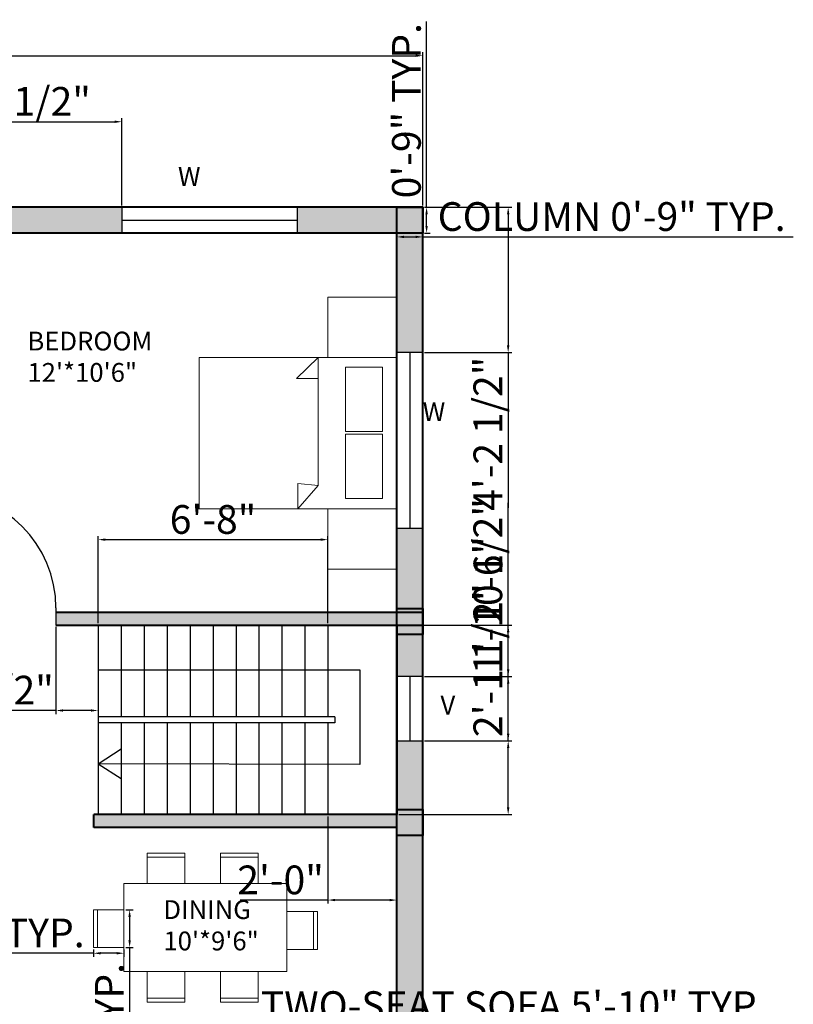
# Model space of a CAD drawing. Units: inches. Extents: x 1628 to 2197, y 2073 to 2736.
# Tile 3 of 3: x 1913 to 2182, y 2323 to 2666. Entities that reach past the tile are written whole.
import ezdxf

# ---------------------------------------------------------------- set-up
doc = ezdxf.new("R2010")
doc.units = ezdxf.units.IN
for name, color, linetype, lineweight in [('A-ANNO-DIMS', 2, 'Continuous', 18), ('A-ANNO-IDEN', 7, 'Continuous', 18), ('A-AREA-IDEN', 7, 'Continuous', 18), ('A-COLS', 7, 'Continuous', 40), ('A-COLS-PATT', 8, 'Continuous', 13), ('A-FLOR-STRS', 7, 'Continuous', 25), ('A-FURN', 8, 'Continuous', 18), ('A-WALL-PATT', 152, 'Continuous', 13), ('bed', 210, 'Continuous', 18), ('door', 52, 'Continuous', 25), ('wall', 151, 'Continuous', 40), ('window', 20, 'Continuous', 25)]:
    doc.layers.add(name, color=color, linetype=linetype, lineweight=lineweight)
doc.styles.get("Standard").update_dxf_attribs({"font": 'arial.ttf'})
doc.dimstyles.new('ISO-25', dxfattribs={"dimtxt": 10, "dimasz": 2.5, "dimexe": 1.25, "dimexo": 0.625, "dimtad": 1, "dimdec": 0, "dimlunit": 4, "dimtxsty": 'Standard', "dimcen": 2.5, "dimadec": 0, "dimazin": 0, "dimtfac": 1, "dimtdec": 0, "dimtmove": 0, "dimatfit": 3, "dimfxl": 1, "dimarcsym": 0})

# ---------------------------------------------------------------- blocks, each defined once
blk = doc.blocks.new('*U2')
for p, q in [((0, 0), (0, -6)), ((40, 0), (40, -6))]:
    blk.add_line(p, q)
blk.add_lwpolyline([(0, 0), (0, 40), (1.75, 40), (1.75, 0)], close=True)
blk.add_arc((0, 0), 40, 0, 90)
blk = doc.blocks.new('*D5')
at = {"layer": 'A-ANNO-DIMS', "color": 0, "lineweight": -2, "transparency": 16777216}
for p, q in [((1693.11, 2601.33), (1693.11, 2654.69)), ((2053.11, 2601.33), (2053.11, 2654.69)), ((1695.61, 2653.44), (2050.61, 2653.44))]:
    blk.add_line(p, q, dxfattribs=at)
at = {"layer": 'A-ANNO-DIMS', "color": 0, "transparency": 16777216}
for points in [[(1695.61, 2653.85), (1695.61, 2653.02), (1693.11, 2653.44)], [(2050.61, 2653.85), (2050.61, 2653.02), (2053.11, 2653.44)]]:
    blk.add_solid(points, dxfattribs=at)
at = {"layer": 'Defpoints', "color": 0, "transparency": 16777216}
for p in [(2053.11, 2653.44), (1693.11, 2600.7), (2053.11, 2600.7)]:
    blk.add_point(p, dxfattribs=at)
at = {"layer": 'A-ANNO-DIMS', "color": 0, "transparency": 16777216, "insert": (1873.11, 2659.17), "char_height": 10, "attachment_point": 5}
blk.add_mtext("30'", dxfattribs=at)
blk = doc.blocks.new('BED-DOUBLE-WITH-NIGHTSTANDS')
for p, q in [((27.37, 65.6), (34.42, 73.72)), ((34.42, 73.72), (34.42, 64.86)), ((27.37, 28.24), (27.37, 65.6)), ((34.42, 64.86), (27.37, 65.6)), ((27.37, 28.24), (27.37, 20.94)), ((27.37, 20.94), (34.96, 28.24)), ((34.96, 28.24), (27.37, 28.24))]:
    blk.add_line(p, q)
for points in [[(0, 73.72), (23.98, 73.72), (23.98, 94.66), (0, 94.66)], [(0, 20.94), (68.84, 20.94), (68.84, 73.72), (0, 73.72)], [(4.97, 47.66), (17.93, 47.66), (17.93, 70.03), (4.97, 70.03)], [(4.97, 24.36), (17.93, 24.36), (17.93, 46.73), (4.97, 46.73)], [(0, 0), (23.98, 0), (23.98, 20.94), (0, 20.94)]]:
    blk.add_lwpolyline(points, close=True)
blk = doc.blocks.new('CHAIR-DINING')
for p, q in [((1.86, 9.22), (0, 9.22)), ((0, 9.22), (13.17, 9.22))]:
    blk.add_line(p, q)
blk.add_lwpolyline([(0, 0), (13.17, 0), (13.17, 10.6), (0, 10.6)], close=True)
blk = doc.blocks.new('WINDOW-61IN')
blk.add_line((0, 4.5), (61.1, 4.5))
blk.add_lwpolyline([(0, 0), (61.1, 0), (61.1, 9), (0, 9)], close=True)
blk = doc.blocks.new('COLUMN-9X9')
blk.add_lwpolyline([(0, 9), (9, 9), (9, 0), (0, 0)], close=True)
blk = doc.blocks.new('*D13')
at = {"layer": 'A-ANNO-DIMS', "color": 0, "lineweight": -2, "transparency": 16777216}
for p, q in [((2044.11, 2591.08), (2044.11, 2589.1)), ((2046.61, 2590.35), (2050.61, 2590.35)), ((2053.11, 2591.08), (2053.11, 2589.1)), ((2053.11, 2590.35), (2182.12, 2590.35))]:
    blk.add_line(p, q, dxfattribs=at)
at = {"layer": 'A-ANNO-DIMS', "color": 0, "transparency": 16777216}
for points in [[(2046.61, 2590.77), (2046.61, 2589.94), (2044.11, 2590.35)], [(2050.61, 2590.77), (2050.61, 2589.94), (2053.11, 2590.35)]]:
    blk.add_solid(points, dxfattribs=at)
at = {"layer": 'Defpoints', "color": 0, "transparency": 16777216}
for p in [(2044.11, 2591.7), (2053.11, 2591.7), (2053.11, 2590.35)]:
    blk.add_point(p, dxfattribs=at)
at = {"layer": 'A-ANNO-DIMS', "color": 0, "transparency": 16777216, "insert": (2118.87, 2596.15), "char_height": 10, "attachment_point": 5}
blk.add_mtext('COLUMN 0\'-9" TYP.', dxfattribs=at)
blk = doc.blocks.new('*D14')
at = {"layer": 'A-ANNO-DIMS', "color": 0, "lineweight": -2, "transparency": 16777216}
for p, q in [((2054.46, 2600.7), (2054.46, 2665.41)), ((2053.74, 2600.7), (2055.71, 2600.7)), ((2054.46, 2594.2), (2054.46, 2598.2)), ((2053.74, 2591.7), (2055.71, 2591.7))]:
    blk.add_line(p, q, dxfattribs=at)
at = {"layer": 'A-ANNO-DIMS', "color": 0, "transparency": 16777216}
for points in [[(2054.04, 2598.2), (2054.88, 2598.2), (2054.46, 2600.7)], [(2054.04, 2594.2), (2054.88, 2594.2), (2054.46, 2591.7)]]:
    blk.add_solid(points, dxfattribs=at)
at = {"layer": 'Defpoints', "color": 0, "transparency": 16777216}
for p in [(2053.11, 2600.7), (2054.46, 2600.7), (2053.11, 2591.7)]:
    blk.add_point(p, dxfattribs=at)
at = {"layer": 'A-ANNO-DIMS', "color": 0, "transparency": 16777216, "insert": (2048.73, 2634.3), "char_height": 10, "attachment_point": 5, "rotation": 90}
blk.add_mtext('0\'-9" TYP.', dxfattribs=at)
blk = doc.blocks.new('*D17')
at = {"layer": 'A-ANNO-DIMS', "color": 0, "lineweight": -2, "transparency": 16777216}
for p, q in [((1949.73, 2356.08), (1952.33, 2356.08)), ((1951.08, 2353.58), (1951.08, 2345.41)), ((1949.73, 2342.91), (1952.33, 2342.91)), ((1951.08, 2342.91), (1951.08, 2230.98))]:
    blk.add_line(p, q, dxfattribs=at)
at = {"layer": 'A-ANNO-DIMS', "color": 0, "transparency": 16777216}
for points in [[(1950.66, 2353.58), (1951.5, 2353.58), (1951.08, 2356.08)], [(1950.66, 2345.41), (1951.5, 2345.41), (1951.08, 2342.91)]]:
    blk.add_solid(points, dxfattribs=at)
at = {"layer": 'Defpoints', "color": 0, "transparency": 16777216}
for p in [(1949.11, 2356.08), (1949.11, 2342.91), (1951.08, 2342.91)]:
    blk.add_point(p, dxfattribs=at)
at = {"layer": 'A-ANNO-DIMS', "color": 0, "transparency": 16777216, "insert": (1945.29, 2285.7), "char_height": 10, "attachment_point": 5, "rotation": 90}
blk.add_mtext('CHAIR 1\'-1" TYP.', dxfattribs=at)
blk = doc.blocks.new('*D18')
at = {"layer": 'A-ANNO-DIMS', "color": 0, "lineweight": -2, "transparency": 16777216}
for p, q in [((1938.5, 2342.29), (1938.5, 2339.69)), ((1949.11, 2342.29), (1949.11, 2339.69)), ((1938.5, 2340.94), (1842.73, 2340.94)), ((1946.61, 2340.94), (1941, 2340.94))]:
    blk.add_line(p, q, dxfattribs=at)
at = {"layer": 'A-ANNO-DIMS', "color": 0, "transparency": 16777216}
for points in [[(1941, 2341.35), (1941, 2340.52), (1938.5, 2340.94)], [(1946.61, 2341.35), (1946.61, 2340.52), (1949.11, 2340.94)]]:
    blk.add_solid(points, dxfattribs=at)
at = {"layer": 'Defpoints', "color": 0, "transparency": 16777216}
for p in [(1938.5, 2342.91), (1949.11, 2342.91), (1938.5, 2340.94)]:
    blk.add_point(p, dxfattribs=at)
at = {"layer": 'A-ANNO-DIMS', "color": 0, "transparency": 16777216, "insert": (1889.36, 2346.73), "char_height": 10, "attachment_point": 5}
blk.add_mtext('0\'-10 1/2" TYP.', dxfattribs=at)
blk = doc.blocks.new('*D23')
at = {"layer": 'A-ANNO-DIMS', "color": 0, "lineweight": -2, "transparency": 16777216}
for p, q in [((1917.57, 2305.72), (1917.57, 2316.85)), ((1920.07, 2315.6), (1985.07, 2315.6)), ((1987.57, 2305.72), (1987.57, 2316.85)), ((1987.57, 2315.6), (2179.82, 2315.6))]:
    blk.add_line(p, q, dxfattribs=at)
at = {"layer": 'A-ANNO-DIMS', "color": 0, "transparency": 16777216}
for points in [[(1920.07, 2316.01), (1920.07, 2315.18), (1917.57, 2315.6)], [(1985.07, 2316.01), (1985.07, 2315.18), (1987.57, 2315.6)]]:
    blk.add_solid(points, dxfattribs=at)
at = {"layer": 'Defpoints', "color": 0, "transparency": 16777216}
for p in [(1987.57, 2315.6), (1917.57, 2305.1), (1987.57, 2305.1)]:
    blk.add_point(p, dxfattribs=at)
at = {"layer": 'A-ANNO-DIMS', "color": 0, "transparency": 16777216, "insert": (2084.94, 2321.4), "char_height": 10, "attachment_point": 5}
blk.add_mtext('TWO-SEAT SOFA 5\'-10" TYP.', dxfattribs=at)
blk = doc.blocks.new('*D24')
at = {"layer": 'A-ANNO-DIMS', "color": 0, "lineweight": -2, "transparency": 16777216}
for p, q in [((1907.07, 2305.1), (1907.07, 2393.27)), ((1916.95, 2305.1), (1905.82, 2305.1)), ((1907.07, 2274.24), (1907.07, 2302.6)), ((1916.95, 2271.74), (1905.82, 2271.74))]:
    blk.add_line(p, q, dxfattribs=at)
at = {"layer": 'A-ANNO-DIMS', "color": 0, "transparency": 16777216}
for points in [[(1906.65, 2302.6), (1907.49, 2302.6), (1907.07, 2305.1)], [(1906.65, 2274.24), (1907.49, 2274.24), (1907.07, 2271.74)]]:
    blk.add_solid(points, dxfattribs=at)
at = {"layer": 'Defpoints', "color": 0, "transparency": 16777216}
for p in [(1907.07, 2305.1), (1917.57, 2305.1), (1917.57, 2271.74)]:
    blk.add_point(p, dxfattribs=at)
at = {"layer": 'A-ANNO-DIMS', "color": 0, "transparency": 16777216, "insert": (1901.28, 2350.44), "char_height": 10, "attachment_point": 5, "rotation": 90}
blk.add_mtext('2\'-9 1/2" TYP.', dxfattribs=at)
blk = doc.blocks.new('*D27')
at = {"layer": 'A-ANNO-DIMS', "color": 0, "lineweight": -2, "transparency": 16777216}
for p, q in [((1873.11, 2592.33), (1873.11, 2631.7)), ((1875.61, 2630.45), (1945.87, 2630.45)), ((1948.37, 2601.33), (1948.37, 2631.7))]:
    blk.add_line(p, q, dxfattribs=at)
at = {"layer": 'A-ANNO-DIMS', "color": 0, "transparency": 16777216}
for points in [[(1875.61, 2630.87), (1875.61, 2630.04), (1873.11, 2630.45)], [(1945.87, 2630.87), (1945.87, 2630.04), (1948.37, 2630.45)]]:
    blk.add_solid(points, dxfattribs=at)
at = {"layer": 'Defpoints', "color": 0, "transparency": 16777216}
for p in [(1948.37, 2630.45), (1948.37, 2600.7), (1873.11, 2591.7)]:
    blk.add_point(p, dxfattribs=at)
at = {"layer": 'A-ANNO-DIMS', "color": 0, "transparency": 16777216, "insert": (1910.74, 2636.25), "char_height": 10, "attachment_point": 5}
blk.add_mtext('6\'-3 1/2"', dxfattribs=at)
blk = doc.blocks.new('*D42')
at = {"layer": 'A-ANNO-DIMS', "color": 0, "lineweight": -2, "transparency": 16777216}
for p, q in [((2053.74, 2600.7), (2084.11, 2600.7)), ((2082.86, 2598.2), (2082.86, 2552.57)), ((2053.74, 2550.07), (2084.11, 2550.07)), ((2082.86, 2550.07), (2082.86, 2496.04))]:
    blk.add_line(p, q, dxfattribs=at)
at = {"layer": 'A-ANNO-DIMS', "color": 0, "transparency": 16777216}
for points in [[(2082.44, 2598.2), (2083.28, 2598.2), (2082.86, 2600.7)], [(2082.44, 2552.57), (2083.28, 2552.57), (2082.86, 2550.07)]]:
    blk.add_solid(points, dxfattribs=at)
at = {"layer": 'Defpoints', "color": 0, "transparency": 16777216}
for p in [(2053.11, 2600.7), (2053.11, 2550.07), (2082.86, 2550.07)]:
    blk.add_point(p, dxfattribs=at)
at = {"layer": 'A-ANNO-DIMS', "color": 0, "transparency": 16777216, "insert": (2077.07, 2521.8), "char_height": 10, "attachment_point": 5, "rotation": 90}
blk.add_mtext('4\'-2 1/2"', dxfattribs=at)
blk = doc.blocks.new('*D43')
at = {"layer": 'A-ANNO-DIMS', "color": 0, "lineweight": -2, "transparency": 16777216}
for p, q in [((2082.86, 2414.88), (2082.86, 2468.69)), ((2053.74, 2414.88), (2084.11, 2414.88)), ((2082.86, 2391.7), (2082.86, 2412.38)), ((2044.74, 2389.2), (2084.11, 2389.2))]:
    blk.add_line(p, q, dxfattribs=at)
at = {"layer": 'A-ANNO-DIMS', "color": 0, "transparency": 16777216}
for points in [[(2082.44, 2412.38), (2083.28, 2412.38), (2082.86, 2414.88)], [(2082.44, 2391.7), (2083.28, 2391.7), (2082.86, 2389.2)]]:
    blk.add_solid(points, dxfattribs=at)
at = {"layer": 'Defpoints', "color": 0, "transparency": 16777216}
for p in [(2053.11, 2414.88), (2082.86, 2414.88), (2044.11, 2389.2)]:
    blk.add_point(p, dxfattribs=at)
at = {"layer": 'A-ANNO-DIMS', "color": 0, "transparency": 16777216, "insert": (2077.07, 2443.03), "char_height": 10, "attachment_point": 5, "rotation": 90}
blk.add_mtext('2\'-1 1/2"', dxfattribs=at)
blk = doc.blocks.new('*D44')
at = {"layer": 'A-ANNO-DIMS', "color": 0, "lineweight": -2, "transparency": 16777216}
for p, q in [((2082.86, 2437.29), (2082.86, 2497.75)), ((2053.74, 2437.29), (2084.11, 2437.29)), ((2082.86, 2417.38), (2082.86, 2434.79)), ((2053.74, 2414.88), (2084.11, 2414.88))]:
    blk.add_line(p, q, dxfattribs=at)
at = {"layer": 'A-ANNO-DIMS', "color": 0, "transparency": 16777216}
for points in [[(2082.44, 2434.79), (2083.28, 2434.79), (2082.86, 2437.29)], [(2082.44, 2417.38), (2083.28, 2417.38), (2082.86, 2414.88)]]:
    blk.add_solid(points, dxfattribs=at)
at = {"layer": 'Defpoints', "color": 0, "transparency": 16777216}
for p in [(2053.11, 2437.29), (2082.86, 2437.29), (2053.11, 2414.88)]:
    blk.add_point(p, dxfattribs=at)
at = {"layer": 'A-ANNO-DIMS', "color": 0, "transparency": 16777216, "insert": (2077.07, 2468.77), "char_height": 10, "attachment_point": 5, "rotation": 90}
blk.add_mtext('1\'-10 1/2"', dxfattribs=at)
blk = doc.blocks.new('*D45')
at = {"layer": 'A-ANNO-DIMS', "color": 0, "lineweight": -2, "transparency": 16777216}
for p, q in [((2082.86, 2455.2), (2082.86, 2484.59)), ((2044.74, 2455.2), (2084.11, 2455.2)), ((2082.86, 2439.79), (2082.86, 2452.7)), ((2053.74, 2437.29), (2084.11, 2437.29))]:
    blk.add_line(p, q, dxfattribs=at)
at = {"layer": 'A-ANNO-DIMS', "color": 0, "transparency": 16777216}
for points in [[(2082.44, 2452.7), (2083.28, 2452.7), (2082.86, 2455.2)], [(2082.44, 2439.79), (2083.28, 2439.79), (2082.86, 2437.29)]]:
    blk.add_solid(points, dxfattribs=at)
at = {"layer": 'Defpoints', "color": 0, "transparency": 16777216}
for p in [(2044.11, 2455.2), (2082.86, 2455.2), (2053.11, 2437.29)]:
    blk.add_point(p, dxfattribs=at)
at = {"layer": 'A-ANNO-DIMS', "color": 0, "transparency": 16777216, "insert": (2077.13, 2471.15), "char_height": 10, "attachment_point": 5, "rotation": 90}
blk.add_mtext('1\'-6"', dxfattribs=at)
blk = doc.blocks.new('*D46')
at = {"layer": 'A-ANNO-DIMS', "color": 0, "lineweight": -2, "transparency": 16777216}
for p, q in [((1940.11, 2455.83), (1940.11, 2486.2)), ((2020.11, 2455.83), (2020.11, 2486.2)), ((1942.61, 2484.95), (2017.61, 2484.95))]:
    blk.add_line(p, q, dxfattribs=at)
at = {"layer": 'A-ANNO-DIMS', "color": 0, "transparency": 16777216}
for points in [[(1942.61, 2485.37), (1942.61, 2484.54), (1940.11, 2484.95)], [(2017.61, 2485.37), (2017.61, 2484.54), (2020.11, 2484.95)]]:
    blk.add_solid(points, dxfattribs=at)
at = {"layer": 'Defpoints', "color": 0, "transparency": 16777216}
for p in [(2020.11, 2484.95), (1940.11, 2455.2), (2020.11, 2455.2)]:
    blk.add_point(p, dxfattribs=at)
at = {"layer": 'A-ANNO-DIMS', "color": 0, "transparency": 16777216, "insert": (1980.11, 2490.68), "char_height": 10, "attachment_point": 5}
blk.add_mtext('6\'-8"', dxfattribs=at)
blk = doc.blocks.new('*D47')
at = {"layer": 'A-ANNO-DIMS', "color": 0, "lineweight": -2, "transparency": 16777216}
for p, q in [((2020.11, 2388.58), (2020.11, 2358.2)), ((2044.11, 2388.58), (2044.11, 2358.2)), ((2020.11, 2359.45), (1989.61, 2359.45)), ((2041.61, 2359.45), (2022.61, 2359.45))]:
    blk.add_line(p, q, dxfattribs=at)
at = {"layer": 'A-ANNO-DIMS', "color": 0, "transparency": 16777216}
for points in [[(2022.61, 2359.87), (2022.61, 2359.04), (2020.11, 2359.45)], [(2041.61, 2359.87), (2041.61, 2359.04), (2044.11, 2359.45)]]:
    blk.add_solid(points, dxfattribs=at)
at = {"layer": 'Defpoints', "color": 0, "transparency": 16777216}
for p in [(2020.11, 2389.2), (2044.11, 2389.2), (2020.11, 2359.45)]:
    blk.add_point(p, dxfattribs=at)
at = {"layer": 'A-ANNO-DIMS', "color": 0, "transparency": 16777216, "insert": (2003.61, 2365.18), "char_height": 10, "attachment_point": 5}
blk.add_mtext('2\'-0"', dxfattribs=at)
blk = doc.blocks.new('*D51')
at = {"layer": 'A-ANNO-DIMS', "color": 0, "lineweight": -2, "transparency": 16777216}
for p, q in [((1925.43, 2454.58), (1925.43, 2424.2)), ((1940.11, 2454.58), (1940.11, 2424.2)), ((1925.43, 2425.45), (1872.74, 2425.45)), ((1937.61, 2425.45), (1927.93, 2425.45))]:
    blk.add_line(p, q, dxfattribs=at)
at = {"layer": 'A-ANNO-DIMS', "color": 0, "transparency": 16777216}
for points in [[(1927.93, 2425.87), (1927.93, 2425.04), (1925.43, 2425.45)], [(1937.61, 2425.87), (1937.61, 2425.04), (1940.11, 2425.45)]]:
    blk.add_solid(points, dxfattribs=at)
at = {"layer": 'Defpoints', "color": 0, "transparency": 16777216}
for p in [(1925.43, 2455.2), (1940.11, 2455.2), (1925.43, 2425.45)]:
    blk.add_point(p, dxfattribs=at)
at = {"layer": 'A-ANNO-DIMS', "color": 0, "transparency": 16777216, "insert": (1897.84, 2431.25), "char_height": 10, "attachment_point": 5}
blk.add_mtext('1\'-2 1/2"', dxfattribs=at)

msp = doc.modelspace()

# ---------------------------------------------------------------- hatches: boundary and pattern name
at = {"layer": 'A-COLS-PATT'}
h = msp.add_hatch(color=256, dxfattribs=at)
h.dxf.hatch_style = 1
h.paths.add_polyline_path([(1702.11, 2600.7), (1693.11, 2600.7), (1693.11, 2591.7), (1702.11, 2591.7)])
h.paths.add_polyline_path([(1879.79, 2600.7), (1870.79, 2600.7), (1870.79, 2591.7), (1879.79, 2591.7)])
h.paths.add_polyline_path([(2053.11, 2600.7), (2044.11, 2600.7), (2044.11, 2591.7), (2053.11, 2591.7)])
h.paths.add_polyline_path([(1702.11, 2395.2), (1693.11, 2395.2), (1693.11, 2386.2), (1702.11, 2386.2)])
h.paths.add_polyline_path([(1826.61, 2395.2), (1817.61, 2395.2), (1817.61, 2386.2), (1826.61, 2386.2)])
h.paths.add_polyline_path([(1702.11, 2459.7), (1693.11, 2459.7), (1693.11, 2450.7), (1702.11, 2450.7)])
h.paths.add_polyline_path([(2053.11, 2459.7), (2044.11, 2459.7), (2044.11, 2455.2), (2053.11, 2455.2)])
h.paths.add_polyline_path([(2053.11, 2455.2), (2044.11, 2455.2), (2044.11, 2451.94), (2053.11, 2451.94)])
h.paths.add_polyline_path([(2053.11, 2460.94), (2044.11, 2460.94), (2044.11, 2459.7), (2053.11, 2459.7)])
h.paths.add_polyline_path([(2053.11, 2390.99), (2044.11, 2390.99), (2044.11, 2381.99), (2053.11, 2381.99)])
h.paths.add_polyline_path([(2053.11, 2322.52), (2044.11, 2322.52), (2044.11, 2313.52), (2053.11, 2313.52)])
h.paths.add_polyline_path([(1702.11, 2294.7), (1693.11, 2294.7), (1693.11, 2285.7), (1702.11, 2285.7)])
h.paths.add_polyline_path([(1702.11, 2129.7), (1693.11, 2129.7), (1693.11, 2120.7), (1702.11, 2120.7)])
h.paths.add_polyline_path([(1831.35, 2129.7), (1822.35, 2129.7), (1822.35, 2120.7), (1831.35, 2120.7)])
h.paths.add_polyline_path([(1883.72, 2129.7), (1874.72, 2129.7), (1874.72, 2120.7), (1883.72, 2120.7)])
h.paths.add_polyline_path([(2053.11, 2129.7), (2044.11, 2129.7), (2044.11, 2120.7), (2053.11, 2120.7)])
at = {"layer": 'A-WALL-PATT'}
h = msp.add_hatch(color=256, dxfattribs=at)
h.dxf.hatch_style = 1
h.paths.add_polyline_path([(1753.01, 2600.7), (1702.11, 2600.7), (1702.11, 2591.7), (1753.01, 2591.7)])
h.paths.add_polyline_path([(1870.79, 2600.7), (1814.12, 2600.7), (1814.12, 2591.7), (1870.79, 2591.7)])
h.paths.add_polyline_path([(1948.37, 2600.7), (1879.79, 2600.7), (1879.79, 2591.7), (1909.32, 2591.7), (1948.37, 2591.7)])
h.paths.add_polyline_path([(2044.11, 2600.7), (2009.47, 2600.7), (2009.47, 2591.7), (2044.11, 2591.7)])
h.paths.add_polyline_path([(2053.11, 2591.7), (2044.11, 2591.7), (2044.11, 2550.07), (2053.11, 2550.07)])
h.paths.add_polyline_path([(1702.11, 2591.7), (1693.11, 2591.7), (1693.11, 2549.95), (1702.11, 2549.95)])
h.paths.add_polyline_path([(1702.11, 2488.85), (1693.11, 2488.85), (1693.11, 2459.7), (1702.11, 2459.7)])
h.paths.add_polyline_path([(1828.05, 2459.7), (1702.11, 2459.7), (1702.11, 2455.2), (1733.61, 2455.2), (1792.11, 2455.2), (1828.05, 2455.2)])
h.paths.add_polyline_path([(1885.43, 2459.7), (1868.05, 2459.7), (1868.05, 2455.2), (1885.43, 2455.2)])
h.paths.add_polyline_path([(2053.11, 2488.97), (2044.11, 2488.97), (2044.11, 2474.68), (2044.11, 2460.94), (2053.11, 2460.94)])
h.paths.add_polyline_path([(2053.11, 2451.94), (2044.11, 2451.94), (2044.11, 2437.29), (2053.11, 2437.29)])
h.paths.add_polyline_path([(2053.11, 2414.88), (2044.11, 2414.88), (2044.11, 2390.99), (2053.11, 2390.99)])
h.paths.add_polyline_path([(2044.11, 2459.7), (1925.43, 2459.7), (1925.43, 2455.2), (2044.11, 2455.2)])
h.paths.add_polyline_path([(2053.11, 2381.99), (2044.11, 2381.99), (2044.11, 2322.52), (2053.11, 2322.52)])
h.paths.add_polyline_path([(1919.51, 2129.7), (1883.72, 2129.7), (1883.72, 2120.7), (1919.51, 2120.7)])
h.paths.add_polyline_path([(2044.11, 2129.7), (1980.61, 2129.7), (1980.61, 2120.7), (2044.11, 2120.7)])
h.paths.add_polyline_path([(2053.11, 2207.91), (2044.11, 2207.91), (2044.11, 2129.7), (2053.11, 2129.7)])
h.paths.add_polyline_path([(2053.11, 2313.52), (2044.11, 2313.52), (2044.11, 2269.02), (2053.11, 2269.02)])
h.paths.add_polyline_path([(1822.35, 2129.7), (1785.25, 2129.7), (1785.25, 2120.7), (1822.35, 2120.7)])
h.paths.add_polyline_path([(1724.14, 2129.7), (1702.11, 2129.7), (1702.11, 2120.7), (1724.14, 2120.7)])
h.paths.add_polyline_path([(1702.11, 2168.74), (1693.11, 2168.74), (1693.11, 2129.7), (1702.11, 2129.7)])
h.paths.add_polyline_path([(1702.11, 2285.7), (1693.11, 2285.7), (1693.11, 2229.84), (1702.11, 2229.84)])
h.paths.add_polyline_path([(1702.11, 2317.65), (1693.11, 2317.65), (1693.11, 2294.7), (1702.11, 2294.7)])
h.paths.add_polyline_path([(1702.11, 2386.2), (1693.11, 2386.2), (1693.11, 2378.75), (1702.11, 2378.75)])
h.paths.add_polyline_path([(2044.11, 2389.2), (1938.65, 2389.2), (1938.65, 2384.7), (2044.11, 2384.7)])
h.paths.add_polyline_path([(1817.61, 2395.2), (1782.07, 2395.2), (1702.11, 2395.2), (1702.11, 2390.7), (1796.61, 2390.7), (1817.61, 2390.7)])
h.paths.add_polyline_path([(1796.61, 2397.27), (1792.11, 2397.27), (1792.11, 2395.2), (1796.61, 2395.2)])
h.paths.add_polyline_path([(1826.61, 2386.2), (1822.11, 2386.2), (1822.11, 2339.52), (1826.61, 2339.52)])
h.paths.add_polyline_path([(1826.61, 2299.52), (1822.11, 2299.52), (1822.11, 2294.7), (1822.11, 2290.2), (1826.61, 2290.2)])
h.paths.add_polyline_path([(1826.61, 2290.2), (1822.11, 2290.2), (1822.11, 2285.08), (1826.61, 2285.08)])
h.paths.add_polyline_path([(1822.11, 2294.7), (1702.11, 2294.7), (1702.11, 2290.2), (1770.51, 2290.2), (1822.11, 2290.2)])
h.paths.add_polyline_path([(1693.11, 2437.86), (1702.11, 2437.86), (1702.11, 2450.7), (1693.11, 2450.7)])
h.paths.add_polyline_path([(1702.11, 2410.6), (1693.11, 2410.6), (1693.11, 2395.2), (1702.11, 2395.2)])

# ---------------------------------------------------------------- linework, layer by layer
at = {"layer": 'A-FLOR-STRS'}
for p, q in [((1940.11, 2455.2), (1940.11, 2389.2)), ((1948.11, 2455.2), (1948.11, 2423.2)), ((1956.11, 2455.2), (1956.11, 2423.2)), ((1964.11, 2455.2), (1964.11, 2423.2)), ((1972.11, 2455.2), (1972.11, 2423.2)), ((1980.11, 2455.2), (1980.11, 2423.2)), ((1988.11, 2455.2), (1988.11, 2423.2)), ((1996.11, 2455.2), (1996.11, 2423.2)), ((2004.11, 2455.2), (2004.11, 2423.2)), ((2012.11, 2455.2), (2012.11, 2423.2)), ((2020.11, 2455.2), (2020.11, 2423.2)), ((1940.11, 2439.57), (2031.26, 2439.57)), ((2031.26, 2439.57), (2031.26, 2406.64)), ((2022.57, 2423.2), (1940.11, 2423.2)), ((2022.57, 2421.2), (1940.11, 2421.2)), ((1948.11, 2421.2), (1948.11, 2389.2)), ((1956.11, 2421.2), (1956.11, 2389.2)), ((1964.11, 2421.2), (1964.11, 2389.2)), ((1972.11, 2421.2), (1972.11, 2389.2)), ((1980.11, 2421.2), (1980.11, 2389.2)), ((1988.11, 2421.2), (1988.11, 2389.2)), ((1996.11, 2421.2), (1996.11, 2389.2)), ((2004.11, 2421.2), (2004.11, 2389.2)), ((2012.11, 2421.2), (2012.11, 2389.2)), ((2020.11, 2421.2), (2020.11, 2389.2)), ((2022.57, 2423.2), (2022.57, 2421.2)), ((1940.11, 2406.94), (1948.11, 2412.13)), ((2031.26, 2406.64), (1940.11, 2406.94)), ((1940.11, 2406.94), (1948.11, 2401.75))]:
    msp.add_line(p, q, dxfattribs=at)
at = {"layer": 'A-FURN'}
msp.add_lwpolyline([(1949.11, 2365.19), (2005.86, 2365.19), (2005.86, 2334.55), (1949.11, 2334.55)], close=True, dxfattribs=at)
at = {"layer": 'wall'}
for p, q in [((1925.43, 2459.7), (2053.11, 2459.7)), ((1925.43, 2455.2), (2053.11, 2455.2)), ((2044.11, 2455.2), (2044.11, 2389.2)), ((2044.11, 2389.2), (1938.65, 2389.2)), ((1938.65, 2384.7), (1938.65, 2389.2)), ((2044.11, 2384.7), (1938.65, 2384.7))]:
    msp.add_line(p, q, dxfattribs=at)
for points in [[(1873.23, 2120.7), (2053.11, 2120.7), (2053.11, 2600.7), (1693.11, 2600.7), (1693.11, 2120.7), (1833.23, 2120.7)], [(1873.11, 2129.7), (2044.11, 2129.7), (2044.11, 2591.7), (1702.11, 2591.7), (1702.11, 2129.7), (1834.98, 2129.7)]]:
    msp.add_lwpolyline(points, dxfattribs=at)
at = {"layer": 'window'}
msp.add_line((2048.61, 2437.29), (2048.61, 2414.88), dxfattribs=at)
msp.add_lwpolyline([(2044.11, 2437.29), (2044.11, 2414.88), (2053.11, 2414.88), (2053.11, 2437.29)], close=True, dxfattribs=at)

# ---------------------------------------------------------------- block references
at = {"layer": 'A-COLS'}
for p in [(2044.11, 2591.7), (2044.11, 2451.94), (2044.11, 2381.99)]:
    msp.add_blockref('COLUMN-9X9', p, dxfattribs=at)
at = {"layer": 'A-FURN'}
for p in [(1957.14, 2365.19), (1982.68, 2365.19)]:
    msp.add_blockref('CHAIR-DINING', p, dxfattribs=at)
at = {"layer": 'A-FURN', "extrusion": (0, 0, -1), "zscale": -1}
for p, rotation in [((-1949.11, 2356.08), 269.9999999999981), ((-1957.14, 2334.55), 180), ((-1982.68, 2334.55), 180)]:
    msp.add_blockref('CHAIR-DINING', p, dxfattribs=dict(at, rotation=rotation))
at = {"layer": 'A-FURN', "rotation": 269.9999999999981}
msp.add_blockref('CHAIR-DINING', (2005.86, 2355.43), dxfattribs=at)
at = {"layer": 'bed', "rotation": 180}
msp.add_blockref('BED-DOUBLE-WITH-NIGHTSTANDS', (2044.11, 2569.34), dxfattribs=at)
at = {"layer": 'door'}
msp.add_blockref('*U2', (1885.43, 2461.2), dxfattribs=at)
at = {"layer": 'window'}
msp.add_blockref('WINDOW-61IN', (1948.37, 2591.7), dxfattribs=at)
at = {"layer": 'window', "rotation": 270.0000000000007}
msp.add_blockref('WINDOW-61IN', (2044.11, 2550.07), dxfattribs=at)

# ---------------------------------------------------------------- texts
at = {"layer": 'A-ANNO-IDEN', "char_height": 6.55, "attachment_point": 1}
for s, insert in [('W', (1967.91, 2614.68)), ('W', (2053.11, 2532.77)), ('V', (2059.29, 2430.61))]:
    msp.add_mtext_dynamic_manual_height_columns(s, width=86.8171, gutter_width=32.74, heights=[0], dxfattribs=dict(at, insert=insert))
at = {"layer": 'A-AREA-IDEN', "char_height": 6.549, "attachment_point": 1}
for s, insert in [('BEDROOM\\P12\'*10\'6"', (1915.51, 2557.36)), ('DINING\\P10\'*9\'6"', (1962.84, 2359.4))]:
    msp.add_mtext_dynamic_manual_height_columns(s, width=86.8171, gutter_width=32.74, heights=[0], dxfattribs=dict(at, insert=insert))

# ---------------------------------------------------------------- dimensions: what is measured, and where the dimension line sits
at = {"layer": 'A-ANNO-DIMS'}
for base, p1, p2, override, picture, middle in [((2053.11, 2653.44), (1693.11, 2600.7), (2053.11, 2600.7), {"dimclrd": 0, "dimclre": 0, "dimclrt": 0}, '*D5', (1873.11, 2659.17)), ((1948.37, 2630.45), (1873.11, 2591.7), (1948.37, 2600.7), {"dimdec": 1, "dimlfac": 1, "dimrnd": 0, "dimzin": 1, "dimdsep": 46, "dimlunit": 4, "dimfrac": 2}, '*D27', (1910.74, 2636.25)), ((2020.11, 2484.95), (1940.11, 2455.2), (2020.11, 2455.2), {"dimdec": 1, "dimlfac": 1, "dimrnd": 0, "dimzin": 1, "dimdsep": 46, "dimlunit": 4, "dimfrac": 2}, '*D46', (1980.11, 2490.68))]:
    dim = msp.add_linear_dim(base=base, p1=p1, p2=p2, dimstyle='ISO-25', override=override, dxfattribs=at)
    dim.commit()
    dim.dimension.update_dxf_attribs({"geometry": picture, "text_midpoint": middle})
for base, p1, p2, angle, text, picture, middle in [((2054.46, 2600.7), (2053.11, 2591.7), (2053.11, 2600.7), 90, '<> TYP.', '*D14', (2048.73, 2634.3)), ((1907.07, 2305.1), (1917.57, 2271.74), (1917.57, 2305.1), 90, '<> TYP.', '*D24', (1901.28, 2350.44)), ((1938.5, 2340.94), (1949.11, 2342.91), (1938.5, 2342.91), 180, '<> TYP.', '*D18', (1889.36, 2346.73)), ((1951.08, 2342.91), (1949.11, 2356.08), (1949.11, 2342.91), 270, 'CHAIR <> TYP.', '*D17', (1945.29, 2285.7))]:
    dim = msp.add_linear_dim(base=base, p1=p1, p2=p2, angle=angle, text=text, dimstyle='ISO-25', override={"dimdec": 1, "dimlfac": 1, "dimrnd": 0, "dimzin": 1, "dimdsep": 46, "dimlunit": 4, "dimfrac": 2}, dxfattribs=at)
    dim.commit()
    dim.dimension.update_dxf_attribs({"geometry": picture, "text_midpoint": middle})
for base, p1, p2, text, picture, middle in [((2053.11, 2590.35), (2044.11, 2591.7), (2053.11, 2591.7), 'COLUMN <> TYP.', '*D13', (2118.87, 2596.15)), ((1987.57, 2315.6), (1917.57, 2305.1), (1987.57, 2305.1), 'TWO-SEAT SOFA <> TYP.', '*D23', (2084.94, 2321.4))]:
    dim = msp.add_linear_dim(base=base, p1=p1, p2=p2, text=text, dimstyle='ISO-25', override={"dimdec": 1, "dimlfac": 1, "dimrnd": 0, "dimzin": 1, "dimdsep": 46, "dimlunit": 4, "dimfrac": 2}, dxfattribs=at)
    dim.commit()
    dim.dimension.update_dxf_attribs({"geometry": picture, "text_midpoint": middle})
for base, p1, p2, angle, picture, middle in [((2082.86, 2550.07), (2053.11, 2600.7), (2053.11, 2550.07), 90, '*D42', (2077.07, 2521.8)), ((2082.86, 2437.29), (2053.11, 2414.88), (2053.11, 2437.29), 90, '*D44', (2077.07, 2468.77)), ((2082.86, 2455.2), (2053.11, 2437.29), (2044.11, 2455.2), 90, '*D45', (2077.13, 2471.15)), ((2082.86, 2414.88), (2044.11, 2389.2), (2053.11, 2414.88), 90, '*D43', (2077.07, 2443.03)), ((1925.43, 2425.45), (1940.11, 2455.2), (1925.43, 2455.2), 180, '*D51', (1897.84, 2431.25)), ((2020.11, 2359.45), (2044.11, 2389.2), (2020.11, 2389.2), 180, '*D47', (2003.61, 2365.18))]:
    dim = msp.add_linear_dim(base=base, p1=p1, p2=p2, angle=angle, dimstyle='ISO-25', override={"dimdec": 1, "dimlfac": 1, "dimrnd": 0, "dimzin": 1, "dimdsep": 46, "dimlunit": 4, "dimfrac": 2}, dxfattribs=at)
    dim.commit()
    dim.dimension.update_dxf_attribs({"geometry": picture, "text_midpoint": middle})

doc.saveas('drawing.dxf')
